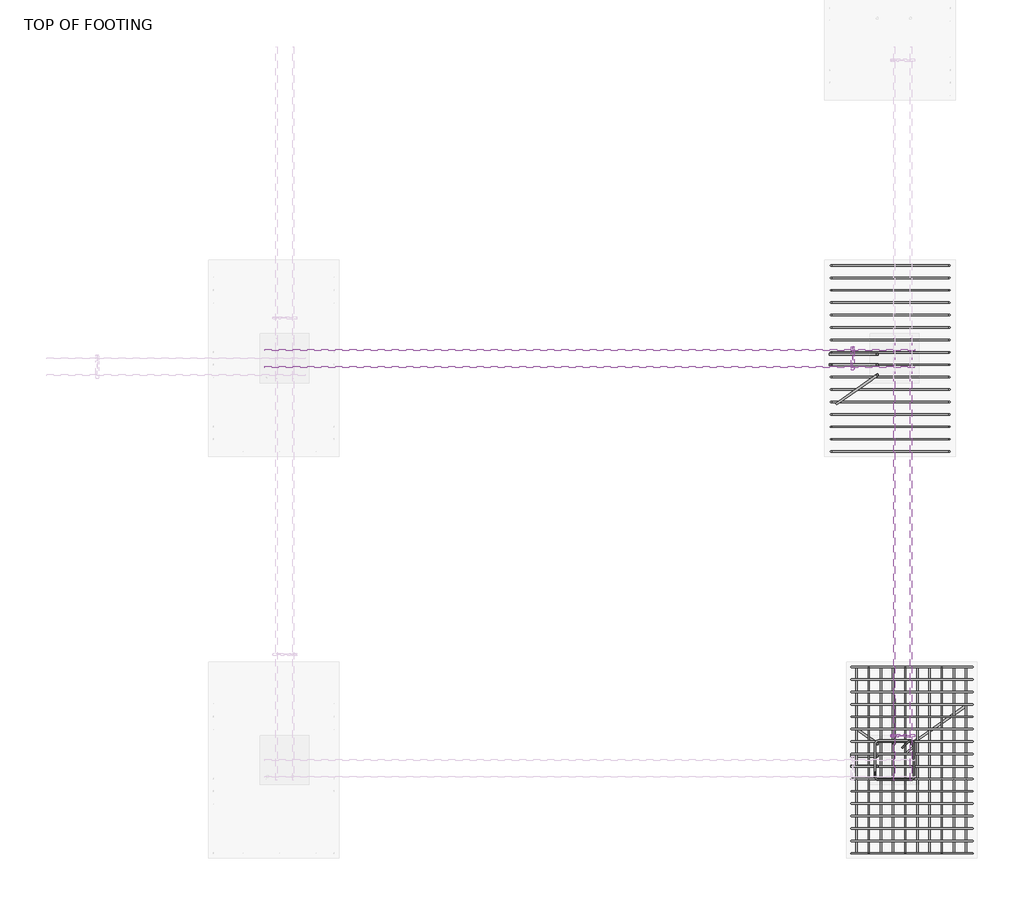
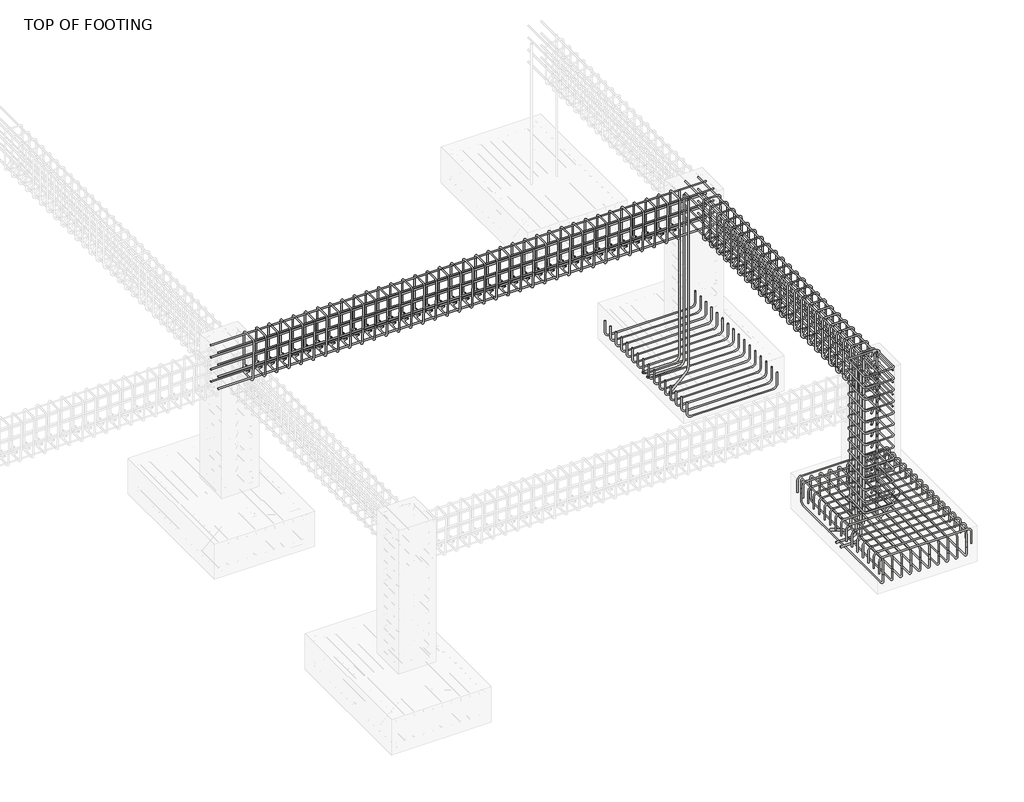
# One storey, part 5 of 11: 17 reinforcing bars.
"""IFC4 building model written with IfcOpenShell, lengths in millimetres."""

from ifc_helpers import new_model, si_unit, point, frame, origin, place, context, project, spatial, polyline, circle_curve, trimmed, segment, composite_curve, source, transform, mapped, element, save
from ifc_brep_helpers import swept_disk

model = new_model("IFC4")

# Units and contexts
model_context = context("Model", 3, world=origin())
ifc_project = project(units=[si_unit("LENGTHUNIT", "METRE", prefix="MILLI")], contexts=[model_context])

# Site, building, storey
site = spatial("IfcSite", under=ifc_project)
building = spatial("IfcBuilding", under=site)
storey = spatial("IfcBuildingStorey", under=building, Name="TOP OF FOOTING", Elevation=-1828.8)

# Reinforcing bars
placement = place(None, origin())
reinforcing_bar_shape = source(origin(), model_context, "Body", "SolidModel", [
    swept_disk(composite_curve([segment(polyline([(2940.9771951, -6018.1250095, -2061.9958198), (2940.9771951, -6018.1250095, -1914.6958198)]), True, "CONTINUOUS"), segment(trimmed(circle_curve(frame((2987.3271951, -6018.1250095, -1914.6958198), z_axis=(0.0, 1.0, 0.0), x_axis=(-46.350000000000364, 0.0, 0.0)), 46.35), [point((2940.9771951, -6018.1250095, -1914.6958198))], [point((2987.3271951, -6018.1250095, -1868.3458198))], True, "CARTESIAN"), True, "CONTINUOUS"), segment(polyline([(2987.3271951, -6018.1250095, -1868.3458198), (4001.9271951, -6018.1250095, -1868.3458198)]), True, "CONTINUOUS"), segment(trimmed(circle_curve(frame((4001.9271951, -6018.1250095, -1914.6958198), z_axis=(0.0, 1.0, 0.0), x_axis=(0.0, 0.0, 46.34999999999991)), 46.35), [point((4001.9271951, -6018.1250095, -1868.3458198))], [point((4048.2771951, -6018.1250095, -1914.6958198))], True, "CARTESIAN"), True, "CONTINUOUS"), segment(polyline([(4048.2771951, -6018.1250095, -1914.6958198), (4048.2771951, -6018.1250095, -2061.9958198)]), True, "CONTINUOUS")], self_intersect=False), 6.35),
])
element("IfcReinforcingBar", 1, at=placement, inside=storey, context=model_context, shape_type="MappedRepresentation", body=[
    mapped(reinforcing_bar_shape, transform((0.0, 0.0, 0.0), x_axis=(1.0, 0.0, 0.0), y_axis=(0.0, 1.0, 0.0), z_axis=(0.0, 0.0, 1.0))),
    mapped(reinforcing_bar_shape, transform((0.0, -113.82, 0.0), x_axis=(1.0, 0.0, 0.0), y_axis=(0.0, 1.0, 0.0), z_axis=(0.0, 0.0, 1.0))),
    mapped(reinforcing_bar_shape, transform((0.0, -227.64, 0.0), x_axis=(1.0, 0.0, 0.0), y_axis=(0.0, 1.0, 0.0), z_axis=(0.0, 0.0, 1.0))),
    mapped(reinforcing_bar_shape, transform((0.0, -341.46, 0.0), x_axis=(1.0, 0.0, 0.0), y_axis=(0.0, 1.0, 0.0), z_axis=(0.0, 0.0, 1.0))),
    mapped(reinforcing_bar_shape, transform((0.0, -455.28, 0.0), x_axis=(1.0, 0.0, 0.0), y_axis=(0.0, 1.0, 0.0), z_axis=(0.0, 0.0, 1.0))),
    mapped(reinforcing_bar_shape, transform((0.0, -569.1, 0.0), x_axis=(1.0, 0.0, 0.0), y_axis=(0.0, 1.0, 0.0), z_axis=(0.0, 0.0, 1.0))),
    mapped(reinforcing_bar_shape, transform((0.0, -682.92, 0.0), x_axis=(1.0, 0.0, 0.0), y_axis=(0.0, 1.0, 0.0), z_axis=(0.0, 0.0, 1.0))),
    mapped(reinforcing_bar_shape, transform((0.0, -796.74, 0.0), x_axis=(1.0, 0.0, 0.0), y_axis=(0.0, 1.0, 0.0), z_axis=(0.0, 0.0, 1.0))),
    mapped(reinforcing_bar_shape, transform((0.0, -910.56, 0.0), x_axis=(1.0, 0.0, 0.0), y_axis=(0.0, 1.0, 0.0), z_axis=(0.0, 0.0, 1.0))),
    mapped(reinforcing_bar_shape, transform((0.0, -1024.38, 0.0), x_axis=(1.0, 0.0, 0.0), y_axis=(0.0, 1.0, 0.0), z_axis=(0.0, 0.0, 1.0))),
    mapped(reinforcing_bar_shape, transform((0.0, -1138.2, 0.0), x_axis=(1.0, 0.0, 0.0), y_axis=(0.0, 1.0, 0.0), z_axis=(0.0, 0.0, 1.0))),
    mapped(reinforcing_bar_shape, transform((0.0, -1252.02, 0.0), x_axis=(1.0, 0.0, 0.0), y_axis=(0.0, 1.0, 0.0), z_axis=(0.0, 0.0, 1.0))),
    mapped(reinforcing_bar_shape, transform((0.0, -1365.84, 0.0), x_axis=(1.0, 0.0, 0.0), y_axis=(0.0, 1.0, 0.0), z_axis=(0.0, 0.0, 1.0))),
    mapped(reinforcing_bar_shape, transform((0.0, -1479.66, 0.0), x_axis=(1.0, 0.0, 0.0), y_axis=(0.0, 1.0, 0.0), z_axis=(0.0, 0.0, 1.0))),
    mapped(reinforcing_bar_shape, transform((0.0, -1593.48, 0.0), x_axis=(1.0, 0.0, 0.0), y_axis=(0.0, 1.0, 0.0), z_axis=(0.0, 0.0, 1.0))),
    mapped(reinforcing_bar_shape, transform((0.0, -1707.3, 0.0), x_axis=(1.0, 0.0, 0.0), y_axis=(0.0, 1.0, 0.0), z_axis=(0.0, 0.0, 1.0))),
])
reinforcing_bar_2_shape = source(origin(), model_context, "Body", "SolidModel", [
    swept_disk(composite_curve([segment(polyline([(3990.0605428, -6018.1250095, -2084.0984403), (3990.0605428, -6018.1250095, -1936.7984403)]), True, "CONTINUOUS"), segment(trimmed(circle_curve(frame((3990.0605428, -6064.4750095, -1936.7984403), z_axis=(1.0, 0.0, 0.0), x_axis=(0.0, 46.350000000000364, 0.0)), 46.35), [point((3990.0605428, -6018.1250095, -1936.7984403))], [point((3990.0605428, -6064.4750095, -1890.4484403))], True, "CARTESIAN"), True, "CONTINUOUS"), segment(polyline([(3990.0605428, -6064.4750095, -1890.4484403), (3990.0605428, -7679.0750095, -1890.4484403)]), True, "CONTINUOUS"), segment(trimmed(circle_curve(frame((3990.0605428, -7679.0750095, -1936.7984403), z_axis=(1.0, 0.0, 0.0), x_axis=(0.0, 0.0, 46.350000000000136)), 46.35), [point((3990.0605428, -7679.0750095, -1890.4484403))], [point((3990.0605428, -7725.4250095, -1936.7984403))], True, "CARTESIAN"), True, "CONTINUOUS"), segment(polyline([(3990.0605428, -7725.4250095, -1936.7984403), (3990.0605428, -7725.4250095, -2084.0984403)]), True, "CONTINUOUS")], self_intersect=False), 6.35),
])
element("IfcReinforcingBar", 2, at=placement, inside=storey, context=model_context, shape_type="MappedRepresentation", body=[
    mapped(reinforcing_bar_2_shape, transform((0.0, 0.0, 0.0), x_axis=(1.0, 0.0, 0.0), y_axis=(0.0, 1.0, 0.0), z_axis=(0.0, 0.0, 1.0))),
    mapped(reinforcing_bar_2_shape, transform((-111.55177, 0.0, 0.0), x_axis=(1.0, 0.0, 0.0), y_axis=(0.0, 1.0, 0.0), z_axis=(0.0, 0.0, 1.0))),
    mapped(reinforcing_bar_2_shape, transform((-223.10354, 0.0, 0.0), x_axis=(1.0, 0.0, 0.0), y_axis=(0.0, 1.0, 0.0), z_axis=(0.0, 0.0, 1.0))),
    mapped(reinforcing_bar_2_shape, transform((-334.6553099, 0.0, 0.0), x_axis=(1.0, 0.0, 0.0), y_axis=(0.0, 1.0, 0.0), z_axis=(0.0, 0.0, 1.0))),
    mapped(reinforcing_bar_2_shape, transform((-446.2070799, 0.0, 0.0), x_axis=(1.0, 0.0, 0.0), y_axis=(0.0, 1.0, 0.0), z_axis=(0.0, 0.0, 1.0))),
    mapped(reinforcing_bar_2_shape, transform((-557.7588499, 0.0, 0.0), x_axis=(1.0, 0.0, 0.0), y_axis=(0.0, 1.0, 0.0), z_axis=(0.0, 0.0, 1.0))),
    mapped(reinforcing_bar_2_shape, transform((-669.3106199, 0.0, 0.0), x_axis=(1.0, 0.0, 0.0), y_axis=(0.0, 1.0, 0.0), z_axis=(0.0, 0.0, 1.0))),
    mapped(reinforcing_bar_2_shape, transform((-780.8623899, 0.0, 0.0), x_axis=(1.0, 0.0, 0.0), y_axis=(0.0, 1.0, 0.0), z_axis=(0.0, 0.0, 1.0))),
    mapped(reinforcing_bar_2_shape, transform((-892.4141599, 0.0, 0.0), x_axis=(1.0, 0.0, 0.0), y_axis=(0.0, 1.0, 0.0), z_axis=(0.0, 0.0, 1.0))),
    mapped(reinforcing_bar_2_shape, transform((-1003.9659298, 0.0, 0.0), x_axis=(1.0, 0.0, 0.0), y_axis=(0.0, 1.0, 0.0), z_axis=(0.0, 0.0, 1.0))),
])
reinforcing_bar_3_shape = source(origin(), model_context, "Body", "SolidModel", [
    swept_disk(composite_curve([segment(polyline([(2986.0946129, -6018.1250095, -2021.5298587), (2986.0946129, -6018.1250095, -2168.8298587)]), True, "CONTINUOUS"), segment(trimmed(circle_curve(frame((2986.0946129, -6064.4750095, -2168.8298587), z_axis=(-1.0, 0.0, 0.0), x_axis=(0.0, 46.350000000000364, 0.0)), 46.35), [point((2986.0946129, -6018.1250095, -2168.8298587))], [point((2986.0946129, -6064.4750095, -2215.1798587))], True, "CARTESIAN"), True, "CONTINUOUS"), segment(polyline([(2986.0946129, -6064.4750095, -2215.1798587), (2986.0946129, -7679.0750095, -2215.1798587)]), True, "CONTINUOUS"), segment(trimmed(circle_curve(frame((2986.0946129, -7679.0750095, -2168.8298587), z_axis=(-1.0, 0.0, 0.0), x_axis=(0.0, 0.0, -46.34999999999991)), 46.35), [point((2986.0946129, -7679.0750095, -2215.1798587))], [point((2986.0946129, -7725.4250095, -2168.8298587))], True, "CARTESIAN"), True, "CONTINUOUS"), segment(polyline([(2986.0946129, -7725.4250095, -2168.8298587), (2986.0946129, -7725.4250095, -2021.5298587)]), True, "CONTINUOUS")], self_intersect=False), 6.35),
])
element("IfcReinforcingBar", 3, at=placement, inside=storey, context=model_context, shape_type="MappedRepresentation", body=[
    mapped(reinforcing_bar_3_shape, transform((0.0, 0.0, 0.0), x_axis=(1.0, 0.0, 0.0), y_axis=(0.0, 1.0, 0.0), z_axis=(0.0, 0.0, 1.0))),
    mapped(reinforcing_bar_3_shape, transform((111.55177, 0.0, 0.0), x_axis=(1.0, 0.0, 0.0), y_axis=(0.0, 1.0, 0.0), z_axis=(0.0, 0.0, 1.0))),
    mapped(reinforcing_bar_3_shape, transform((223.10354, 0.0, 0.0), x_axis=(1.0, 0.0, 0.0), y_axis=(0.0, 1.0, 0.0), z_axis=(0.0, 0.0, 1.0))),
    mapped(reinforcing_bar_3_shape, transform((334.6553099, 0.0, 0.0), x_axis=(1.0, 0.0, 0.0), y_axis=(0.0, 1.0, 0.0), z_axis=(0.0, 0.0, 1.0))),
    mapped(reinforcing_bar_3_shape, transform((446.2070799, 0.0, 0.0), x_axis=(1.0, 0.0, 0.0), y_axis=(0.0, 1.0, 0.0), z_axis=(0.0, 0.0, 1.0))),
    mapped(reinforcing_bar_3_shape, transform((557.7588499, 0.0, 0.0), x_axis=(1.0, 0.0, 0.0), y_axis=(0.0, 1.0, 0.0), z_axis=(0.0, 0.0, 1.0))),
    mapped(reinforcing_bar_3_shape, transform((669.3106199, 0.0, 0.0), x_axis=(1.0, 0.0, 0.0), y_axis=(0.0, 1.0, 0.0), z_axis=(0.0, 0.0, 1.0))),
    mapped(reinforcing_bar_3_shape, transform((780.8623899, 0.0, 0.0), x_axis=(1.0, 0.0, 0.0), y_axis=(0.0, 1.0, 0.0), z_axis=(0.0, 0.0, 1.0))),
    mapped(reinforcing_bar_3_shape, transform((892.4141599, 0.0, 0.0), x_axis=(1.0, 0.0, 0.0), y_axis=(0.0, 1.0, 0.0), z_axis=(0.0, 0.0, 1.0))),
    mapped(reinforcing_bar_3_shape, transform((1003.9659298, 0.0, 0.0), x_axis=(1.0, 0.0, 0.0), y_axis=(0.0, 1.0, 0.0), z_axis=(0.0, 0.0, 1.0))),
])
reinforcing_bar_4_shape = source(origin(), model_context, "Body", "SolidModel", [
    swept_disk(composite_curve([segment(polyline([(3836.7789753, -2335.4013044, -2046.7466921), (3836.7789753, -2335.4013044, -2194.0466921)]), True, "CONTINUOUS"), segment(trimmed(circle_curve(frame((3790.4289753, -2335.4013044, -2194.0466921), z_axis=(0.0, 1.0, 0.0), x_axis=(46.350000000000364, 0.0, 0.0)), 46.35), [point((3836.7789753, -2335.4013044, -2194.0466921))], [point((3790.4289753, -2335.4013044, -2240.3966921))], True, "CARTESIAN"), True, "CONTINUOUS"), segment(polyline([(3790.4289753, -2335.4013044, -2240.3966921), (2799.2007226, -2335.4013044, -2240.3966921)]), True, "CONTINUOUS"), segment(trimmed(circle_curve(frame((2799.2007226, -2335.4013044, -2194.0466921), z_axis=(0.0, 1.0, 0.0), x_axis=(0.0, 0.0, -46.34999999999991)), 46.35), [point((2799.2007226, -2335.4013044, -2240.3966921))], [point((2752.8507226, -2335.4013044, -2194.0466921))], True, "CARTESIAN"), True, "CONTINUOUS"), segment(polyline([(2752.8507226, -2335.4013044, -2194.0466921), (2752.8507226, -2335.4013044, -2046.7466921)]), True, "CONTINUOUS")], self_intersect=False), 6.35),
])
element("IfcReinforcingBar", 4, at=placement, inside=storey, context=model_context, shape_type="MappedRepresentation", body=[
    mapped(reinforcing_bar_4_shape, transform((0.0, 0.0, 0.0), x_axis=(1.0, 0.0, 0.0), y_axis=(0.0, 1.0, 0.0), z_axis=(0.0, 0.0, 1.0))),
    mapped(reinforcing_bar_4_shape, transform((0.0, -113.82, 0.0), x_axis=(1.0, 0.0, 0.0), y_axis=(0.0, 1.0, 0.0), z_axis=(0.0, 0.0, 1.0))),
    mapped(reinforcing_bar_4_shape, transform((0.0, -227.64, 0.0), x_axis=(1.0, 0.0, 0.0), y_axis=(0.0, 1.0, 0.0), z_axis=(0.0, 0.0, 1.0))),
    mapped(reinforcing_bar_4_shape, transform((0.0, -341.46, 0.0), x_axis=(1.0, 0.0, 0.0), y_axis=(0.0, 1.0, 0.0), z_axis=(0.0, 0.0, 1.0))),
    mapped(reinforcing_bar_4_shape, transform((0.0, -455.28, 0.0), x_axis=(1.0, 0.0, 0.0), y_axis=(0.0, 1.0, 0.0), z_axis=(0.0, 0.0, 1.0))),
    mapped(reinforcing_bar_4_shape, transform((0.0, -569.1, 0.0), x_axis=(1.0, 0.0, 0.0), y_axis=(0.0, 1.0, 0.0), z_axis=(0.0, 0.0, 1.0))),
    mapped(reinforcing_bar_4_shape, transform((0.0, -682.92, 0.0), x_axis=(1.0, 0.0, 0.0), y_axis=(0.0, 1.0, 0.0), z_axis=(0.0, 0.0, 1.0))),
    mapped(reinforcing_bar_4_shape, transform((0.0, -796.74, 0.0), x_axis=(1.0, 0.0, 0.0), y_axis=(0.0, 1.0, 0.0), z_axis=(0.0, 0.0, 1.0))),
    mapped(reinforcing_bar_4_shape, transform((0.0, -910.56, 0.0), x_axis=(1.0, 0.0, 0.0), y_axis=(0.0, 1.0, 0.0), z_axis=(0.0, 0.0, 1.0))),
    mapped(reinforcing_bar_4_shape, transform((0.0, -1024.38, 0.0), x_axis=(1.0, 0.0, 0.0), y_axis=(0.0, 1.0, 0.0), z_axis=(0.0, 0.0, 1.0))),
    mapped(reinforcing_bar_4_shape, transform((0.0, -1138.2, 0.0), x_axis=(1.0, 0.0, 0.0), y_axis=(0.0, 1.0, 0.0), z_axis=(0.0, 0.0, 1.0))),
    mapped(reinforcing_bar_4_shape, transform((0.0, -1252.02, 0.0), x_axis=(1.0, 0.0, 0.0), y_axis=(0.0, 1.0, 0.0), z_axis=(0.0, 0.0, 1.0))),
    mapped(reinforcing_bar_4_shape, transform((0.0, -1365.84, 0.0), x_axis=(1.0, 0.0, 0.0), y_axis=(0.0, 1.0, 0.0), z_axis=(0.0, 0.0, 1.0))),
    mapped(reinforcing_bar_4_shape, transform((0.0, -1479.66, 0.0), x_axis=(1.0, 0.0, 0.0), y_axis=(0.0, 1.0, 0.0), z_axis=(0.0, 0.0, 1.0))),
    mapped(reinforcing_bar_4_shape, transform((0.0, -1593.48, 0.0), x_axis=(1.0, 0.0, 0.0), y_axis=(0.0, 1.0, 0.0), z_axis=(0.0, 0.0, 1.0))),
    mapped(reinforcing_bar_4_shape, transform((0.0, -1707.3, 0.0), x_axis=(1.0, 0.0, 0.0), y_axis=(0.0, 1.0, 0.0), z_axis=(0.0, 0.0, 1.0))),
])
reinforcing_bar_5_shape = source(origin(), model_context, "Body", "SolidModel", [
    swept_disk(composite_curve([segment(polyline([(3404.0158346, -6758.0507749, -46.35), (3459.7593975, -6702.3072119, -46.35)]), True, "CONTINUOUS"), segment(trimmed(circle_curve(frame((3481.9271951, -6724.4750095, -46.35), z_axis=(0.0, 0.0, -1.0), x_axis=(-22.167797600000085, 22.167797600000085, 0.0)), 31.35), [point((3459.7593975, -6702.3072119, -46.35))], [point((3513.2771951, -6724.4750095, -46.35))], True, "CARTESIAN"), True, "CONTINUOUS"), segment(polyline([(3513.2771951, -6724.4750095, -46.35), (3513.2771951, -7019.0750095, -46.35)]), True, "CONTINUOUS"), segment(trimmed(circle_curve(frame((3481.9271951, -7019.0750095, -46.35), z_axis=(0.0, 0.0, -1.0), x_axis=(31.34999999999991, 0.0, 0.0)), 31.35), [point((3513.2771951, -7019.0750095, -46.35))], [point((3481.9271951, -7050.4250095, -46.35))], True, "CARTESIAN"), True, "CONTINUOUS"), segment(polyline([(3481.9271951, -7050.4250095, -46.35), (3187.3271951, -7050.4250095, -46.35)]), True, "CONTINUOUS"), segment(trimmed(circle_curve(frame((3187.3271951, -7019.0947946, -45.2363875), z_axis=(0.0, 0.03552192833448212, -0.9993688971583016), x_axis=(0.0, -31.3302149000001, -1.1136125000000021)), 31.35), [point((3187.3271951, -7050.4250095, -46.35))], [point((3155.9771951, -7019.0947946, -45.2363875))], True, "CARTESIAN"), True, "CONTINUOUS"), segment(polyline([(3155.9771951, -7019.0947946, -45.2363875), (3155.9771951, -6724.4552244, -34.7636125)]), True, "CONTINUOUS"), segment(trimmed(circle_curve(frame((3187.3271951, -6724.4552244, -34.7636125), z_axis=(0.0, 0.03552192833448212, -0.9993688971583016), x_axis=(-31.350000000000364, 0.0, 0.0)), 31.35), [point((3155.9771951, -6724.4552244, -34.7636125))], [point((3187.3271951, -6693.1250095, -33.65))], True, "CARTESIAN"), True, "CONTINUOUS"), segment(polyline([(3187.3271951, -6693.1250095, -33.65), (3481.9271951, -6693.1250095, -33.65)]), True, "CONTINUOUS"), segment(trimmed(circle_curve(frame((3481.9271951, -6724.4750095, -33.65), z_axis=(0.0, 0.0, -1.0), x_axis=(0.0, 31.350000000000364, 0.0)), 31.35), [point((3481.9271951, -6693.1250095, -33.65))], [point((3504.0949927, -6746.6428071, -33.65))], True, "CARTESIAN"), True, "CONTINUOUS"), segment(polyline([(3504.0949927, -6746.6428071, -33.65), (3448.3514297, -6802.3863701, -33.65)]), True, "CONTINUOUS")], self_intersect=False), 6.35),
])
element("IfcReinforcingBar", 5, at=placement, inside=storey, context=model_context, shape_type="MappedRepresentation", body=[
    mapped(reinforcing_bar_5_shape, transform((0.0, 0.0, 0.0), x_axis=(1.0, 0.0, 0.0), y_axis=(0.0, 1.0, 0.0), z_axis=(0.0, 0.0, 1.0))),
    mapped(reinforcing_bar_5_shape, transform((0.0, 0.0, -144.675), x_axis=(1.0, 0.0, 0.0), y_axis=(0.0, 1.0, 0.0), z_axis=(0.0, 0.0, 1.0))),
    mapped(reinforcing_bar_5_shape, transform((0.0, 0.0, -289.35), x_axis=(1.0, 0.0, 0.0), y_axis=(0.0, 1.0, 0.0), z_axis=(0.0, 0.0, 1.0))),
    mapped(reinforcing_bar_5_shape, transform((0.0, 0.0, -434.025), x_axis=(1.0, 0.0, 0.0), y_axis=(0.0, 1.0, 0.0), z_axis=(0.0, 0.0, 1.0))),
    mapped(reinforcing_bar_5_shape, transform((0.0, 0.0, -578.7), x_axis=(1.0, 0.0, 0.0), y_axis=(0.0, 1.0, 0.0), z_axis=(0.0, 0.0, 1.0))),
    mapped(reinforcing_bar_5_shape, transform((0.0, 0.0, -723.375), x_axis=(1.0, 0.0, 0.0), y_axis=(0.0, 1.0, 0.0), z_axis=(0.0, 0.0, 1.0))),
    mapped(reinforcing_bar_5_shape, transform((0.0, 0.0, -868.05), x_axis=(1.0, 0.0, 0.0), y_axis=(0.0, 1.0, 0.0), z_axis=(0.0, 0.0, 1.0))),
    mapped(reinforcing_bar_5_shape, transform((0.0, 0.0, -1012.725), x_axis=(1.0, 0.0, 0.0), y_axis=(0.0, 1.0, 0.0), z_axis=(0.0, 0.0, 1.0))),
    mapped(reinforcing_bar_5_shape, transform((0.0, 0.0, -1157.4), x_axis=(1.0, 0.0, 0.0), y_axis=(0.0, 1.0, 0.0), z_axis=(0.0, 0.0, 1.0))),
    mapped(reinforcing_bar_5_shape, transform((0.0, 0.0, -1302.075), x_axis=(1.0, 0.0, 0.0), y_axis=(0.0, 1.0, 0.0), z_axis=(0.0, 0.0, 1.0))),
    mapped(reinforcing_bar_5_shape, transform((0.0, 0.0, -1446.75), x_axis=(1.0, 0.0, 0.0), y_axis=(0.0, 1.0, 0.0), z_axis=(0.0, 0.0, 1.0))),
    mapped(reinforcing_bar_5_shape, transform((0.0, 0.0, -1591.425), x_axis=(1.0, 0.0, 0.0), y_axis=(0.0, 1.0, 0.0), z_axis=(0.0, 0.0, 1.0))),
    mapped(reinforcing_bar_5_shape, transform((0.0, 0.0, -1736.1), x_axis=(1.0, 0.0, 0.0), y_axis=(0.0, 1.0, 0.0), z_axis=(0.0, 0.0, 1.0))),
])
element("IfcReinforcingBar", 6, at=placement, inside=storey, context=model_context, shape_type="SolidModel", body=[
    swept_disk(composite_curve([segment(polyline([(3491.9271951, -6720.8250095, -40.0), (3491.9271951, -6720.8250095, -2136.75)]), True, "CONTINUOUS"), segment(trimmed(circle_curve(frame((3546.8513397, -6682.3667095, -2136.75), z_axis=(0.5735764363510477, -0.8191520442889907, 0.0), x_axis=(-54.92414460000009, -38.458300000000236, 0.0)), 67.05), [point((3491.9271951, -6720.8250095, -2136.75))], [point((3546.8513397, -6682.3667095, -2203.8))], True, "CARTESIAN"), True, "CONTINUOUS"), segment(polyline([(3546.8513397, -6682.3667095, -2203.8), (3989.9912438, -6372.0768081, -2203.8)]), True, "CONTINUOUS")], self_intersect=False), 9.55),
])
element("IfcReinforcingBar", 7, at=placement, inside=storey, context=model_context, shape_type="SolidModel", body=[
    swept_disk(composite_curve([segment(polyline([(3177.3271951, -6720.8250095, -40.0), (3177.3271951, -6720.8250095, -2136.75)]), True, "CONTINUOUS"), segment(trimmed(circle_curve(frame((3122.4030505, -6682.3667095, -2136.75), z_axis=(0.5735764363510478, 0.8191520442889907, 0.0), x_axis=(54.92414460000009, -38.458300000000236, 0.0)), 67.05), [point((3177.3271951, -6720.8250095, -2136.75))], [point((3122.4030505, -6682.3667095, -2203.8))], True, "CARTESIAN"), True, "CONTINUOUS"), segment(polyline([(3122.4030505, -6682.3667095, -2203.8), (2999.2631464, -6596.1432204, -2203.8)]), True, "CONTINUOUS")], self_intersect=False), 9.55),
])
reinforcing_bar_6_shape = source(origin(), model_context, "Body", "SolidModel", [
    swept_disk(composite_curve([segment(polyline([(3177.3271951, -6833.1823983, -40.0), (3177.3271951, -6833.1823983, -2136.75)]), True, "CONTINUOUS"), segment(trimmed(circle_curve(frame((3110.2771951, -6833.1823983, -2136.75), z_axis=(0.0, 1.0, 0.0), x_axis=(67.05000000000018, 0.0, 0.0)), 67.05), [point((3177.3271951, -6833.1823983, -2136.75))], [point((3110.2771951, -6833.1823983, -2203.8))], True, "CARTESIAN"), True, "CONTINUOUS"), segment(polyline([(3110.2771951, -6833.1823983, -2203.8), (2934.6271951, -6833.1823983, -2203.8)]), True, "CONTINUOUS")], self_intersect=False), 9.55),
])
element("IfcReinforcingBar", 8, at=placement, inside=storey, context=model_context, shape_type="MappedRepresentation", body=[
    mapped(reinforcing_bar_6_shape, transform((0.0, 0.0, 0.0), x_axis=(1.0, 0.0, 0.0), y_axis=(0.0, 1.0, 0.0), z_axis=(0.0, 0.0, 1.0))),
    mapped(reinforcing_bar_6_shape, transform((0.0, -94.3634327, 0.0), x_axis=(1.0, 0.0, 0.0), y_axis=(0.0, 1.0, 0.0), z_axis=(0.0, 0.0, 1.0))),
])
element("IfcReinforcingBar", 9, at=placement, inside=storey, context=model_context, shape_type="SolidModel", body=[
    swept_disk(composite_curve([segment(polyline([(3331.9271951, -6720.8250095, -40.0), (3331.9271951, -6720.8250095, -2136.75)]), True, "CONTINUOUS"), segment(trimmed(circle_curve(frame((3331.9271951, -6653.7750095, -2136.75), z_axis=(1.0, 0.0, 0.0), x_axis=(0.0, -67.05000000000018, 0.0)), 67.05), [point((3331.9271951, -6720.8250095, -2136.75))], [point((3331.9271951, -6653.7750095, -2203.8))], True, "CARTESIAN"), True, "CONTINUOUS"), segment(polyline([(3331.9271951, -6653.7750095, -2203.8), (3331.9271951, -6308.1250095, -2203.8)]), True, "CONTINUOUS")], self_intersect=False), 9.55),
])
element("IfcReinforcingBar", 10, at=placement, inside=storey, context=model_context, shape_type="SolidModel", body=[
    swept_disk(composite_curve([segment(polyline([(3177.3271951, -3340.0013044, -40.0), (3177.3271951, -3340.0013044, -2136.75)]), True, "CONTINUOUS"), segment(trimmed(circle_curve(frame((3122.4030505, -3378.4596044, -2136.75), z_axis=(-0.5735764363510477, 0.8191520442889907, 0.0), x_axis=(54.92414460000009, 38.45829999999978, 0.0)), 67.05), [point((3177.3271951, -3340.0013044, -2136.75))], [point((3122.4030505, -3378.4596044, -2203.8))], True, "CARTESIAN"), True, "CONTINUOUS"), segment(polyline([(3122.4030505, -3378.4596044, -2203.8), (2799.2631464, -3604.7246012, -2203.8)]), True, "CONTINUOUS")], self_intersect=False), 9.55),
])
reinforcing_bar_7_shape = source(origin(), model_context, "Body", "SolidModel", [
    swept_disk(composite_curve([segment(polyline([(3177.3271951, -3150.4586931, -40.0), (3177.3271951, -3150.4586931, -2136.75)]), True, "CONTINUOUS"), segment(trimmed(circle_curve(frame((3110.2771951, -3150.4586931, -2136.75), z_axis=(0.0, 1.0, 0.0), x_axis=(67.05000000000018, 0.0, 0.0)), 67.05), [point((3177.3271951, -3150.4586931, -2136.75))], [point((3110.2771951, -3150.4586931, -2203.8))], True, "CARTESIAN"), True, "CONTINUOUS"), segment(polyline([(3110.2771951, -3150.4586931, -2203.8), (2734.6271951, -3150.4586931, -2203.8)]), True, "CONTINUOUS")], self_intersect=False), 9.55),
])
element("IfcReinforcingBar", 11, at=placement, inside=storey, context=model_context, shape_type="MappedRepresentation", body=[
    mapped(reinforcing_bar_7_shape, transform((0.0, 0.0, 0.0), x_axis=(1.0, 0.0, 0.0), y_axis=(0.0, 1.0, 0.0), z_axis=(0.0, 0.0, 1.0))),
    mapped(reinforcing_bar_7_shape, transform((0.0, -94.3634327, 0.0), x_axis=(1.0, 0.0, 0.0), y_axis=(0.0, 1.0, 0.0), z_axis=(0.0, 0.0, 1.0))),
])
reinforcing_bar_8_shape = source(origin(), model_context, "Body", "SolidModel", [
    swept_disk(composite_curve([segment(polyline([(3415.2385556, -6640.4250095, -488.7242346), (3359.4949927, -6640.4250095, -544.4677976)]), True, "CONTINUOUS"), segment(trimmed(circle_curve(frame((3337.3271951, -6640.4250095, -522.3), z_axis=(0.0, 1.0, 0.0), x_axis=(22.16779759999963, 0.0, -22.167797600000085)), 31.35), [point((3359.4949927, -6640.4250095, -544.4677976))], [point((3305.9771951, -6640.4250095, -522.3))], True, "CARTESIAN"), True, "CONTINUOUS"), segment(polyline([(3305.9771951, -6640.4250095, -522.3), (3305.9771951, -6640.4250095, -77.7)]), True, "CONTINUOUS"), segment(trimmed(circle_curve(frame((3337.3271951, -6640.4250095, -77.7), z_axis=(0.0, 1.0, 0.0), x_axis=(-31.350000000000364, 0.0, 0.0)), 31.35), [point((3305.9771951, -6640.4250095, -77.7))], [point((3337.3271951, -6640.4250095, -46.35))], True, "CARTESIAN"), True, "CONTINUOUS"), segment(polyline([(3337.3271951, -6640.4250095, -46.35), (3481.9271951, -6640.4250095, -46.35)]), True, "CONTINUOUS"), segment(trimmed(circle_curve(frame((3481.9271951, -6641.2095952, -77.6901807), z_axis=(0.0, 0.9996867842138424, -0.025026655153786322), x_axis=(0.0, 0.784585700000207, 31.340180699999998)), 31.35), [point((3481.9271951, -6640.4250095, -46.35))], [point((3513.2771951, -6641.2095952, -77.6901807))], True, "CARTESIAN"), True, "CONTINUOUS"), segment(polyline([(3513.2771951, -6641.2095952, -77.6901807), (3513.2771951, -6652.3404239, -522.3098193)]), True, "CONTINUOUS"), segment(trimmed(circle_curve(frame((3481.9271951, -6652.3404239, -522.3098193), z_axis=(0.0, 0.9996867842138424, -0.025026655153786322), x_axis=(31.34999999999991, 0.0, 0.0)), 31.35), [point((3513.2771951, -6652.3404239, -522.3098193))], [point((3481.9271951, -6653.1250095, -553.65))], True, "CARTESIAN"), True, "CONTINUOUS"), segment(polyline([(3481.9271951, -6653.1250095, -553.65), (3337.3271951, -6653.1250095, -553.65)]), True, "CONTINUOUS"), segment(trimmed(circle_curve(frame((3337.3271951, -6653.1250095, -522.3), z_axis=(0.0, 1.0, 0.0), x_axis=(0.0, 0.0, -31.350000000000023)), 31.35), [point((3337.3271951, -6653.1250095, -553.65))], [point((3315.1593975, -6653.1250095, -500.1322024))], True, "CARTESIAN"), True, "CONTINUOUS"), segment(polyline([(3315.1593975, -6653.1250095, -500.1322024), (3370.9029605, -6653.1250095, -444.3886395)]), True, "CONTINUOUS")], self_intersect=False), 6.35),
])
element("IfcReinforcingBar", 12, at=placement, inside=storey, context=model_context, shape_type="MappedRepresentation", body=[
    mapped(reinforcing_bar_8_shape, transform((0.0, 0.0, 0.0), x_axis=(1.0, 0.0, 0.0), y_axis=(0.0, 1.0, 0.0), z_axis=(0.0, 0.0, 1.0))),
    mapped(reinforcing_bar_8_shape, transform((0.0, 146.3647139, 0.0), x_axis=(1.0, 0.0, 0.0), y_axis=(0.0, 1.0, 0.0), z_axis=(0.0, 0.0, 1.0))),
    mapped(reinforcing_bar_8_shape, transform((0.0, 292.7294277, 0.0), x_axis=(1.0, 0.0, 0.0), y_axis=(0.0, 1.0, 0.0), z_axis=(0.0, 0.0, 1.0))),
    mapped(reinforcing_bar_8_shape, transform((0.0, 439.0941416, 0.0), x_axis=(1.0, 0.0, 0.0), y_axis=(0.0, 1.0, 0.0), z_axis=(0.0, 0.0, 1.0))),
    mapped(reinforcing_bar_8_shape, transform((0.0, 585.4588555, 0.0), x_axis=(1.0, 0.0, 0.0), y_axis=(0.0, 1.0, 0.0), z_axis=(0.0, 0.0, 1.0))),
    mapped(reinforcing_bar_8_shape, transform((0.0, 731.8235693, 0.0), x_axis=(1.0, 0.0, 0.0), y_axis=(0.0, 1.0, 0.0), z_axis=(0.0, 0.0, 1.0))),
    mapped(reinforcing_bar_8_shape, transform((0.0, 878.1882832, 0.0), x_axis=(1.0, 0.0, 0.0), y_axis=(0.0, 1.0, 0.0), z_axis=(0.0, 0.0, 1.0))),
    mapped(reinforcing_bar_8_shape, transform((0.0, 1024.5529971, 0.0), x_axis=(1.0, 0.0, 0.0), y_axis=(0.0, 1.0, 0.0), z_axis=(0.0, 0.0, 1.0))),
    mapped(reinforcing_bar_8_shape, transform((0.0, 1170.917711, 0.0), x_axis=(1.0, 0.0, 0.0), y_axis=(0.0, 1.0, 0.0), z_axis=(0.0, 0.0, 1.0))),
    mapped(reinforcing_bar_8_shape, transform((0.0, 1317.2824248, 0.0), x_axis=(1.0, 0.0, 0.0), y_axis=(0.0, 1.0, 0.0), z_axis=(0.0, 0.0, 1.0))),
    mapped(reinforcing_bar_8_shape, transform((0.0, 1463.6471387, 0.0), x_axis=(1.0, 0.0, 0.0), y_axis=(0.0, 1.0, 0.0), z_axis=(0.0, 0.0, 1.0))),
    mapped(reinforcing_bar_8_shape, transform((0.0, 1610.0118526, 0.0), x_axis=(1.0, 0.0, 0.0), y_axis=(0.0, 1.0, 0.0), z_axis=(0.0, 0.0, 1.0))),
    mapped(reinforcing_bar_8_shape, transform((0.0, 1756.3765664, 0.0), x_axis=(1.0, 0.0, 0.0), y_axis=(0.0, 1.0, 0.0), z_axis=(0.0, 0.0, 1.0))),
    mapped(reinforcing_bar_8_shape, transform((0.0, 1902.7412803, 0.0), x_axis=(1.0, 0.0, 0.0), y_axis=(0.0, 1.0, 0.0), z_axis=(0.0, 0.0, 1.0))),
    mapped(reinforcing_bar_8_shape, transform((0.0, 2049.1059942, 0.0), x_axis=(1.0, 0.0, 0.0), y_axis=(0.0, 1.0, 0.0), z_axis=(0.0, 0.0, 1.0))),
    mapped(reinforcing_bar_8_shape, transform((0.0, 2195.470708, 0.0), x_axis=(1.0, 0.0, 0.0), y_axis=(0.0, 1.0, 0.0), z_axis=(0.0, 0.0, 1.0))),
    mapped(reinforcing_bar_8_shape, transform((0.0, 2341.8354219, 0.0), x_axis=(1.0, 0.0, 0.0), y_axis=(0.0, 1.0, 0.0), z_axis=(0.0, 0.0, 1.0))),
    mapped(reinforcing_bar_8_shape, transform((0.0, 2488.2001358, 0.0), x_axis=(1.0, 0.0, 0.0), y_axis=(0.0, 1.0, 0.0), z_axis=(0.0, 0.0, 1.0))),
    mapped(reinforcing_bar_8_shape, transform((0.0, 2634.5648497, 0.0), x_axis=(1.0, 0.0, 0.0), y_axis=(0.0, 1.0, 0.0), z_axis=(0.0, 0.0, 1.0))),
    mapped(reinforcing_bar_8_shape, transform((0.0, 2780.9295635, 0.0), x_axis=(1.0, 0.0, 0.0), y_axis=(0.0, 1.0, 0.0), z_axis=(0.0, 0.0, 1.0))),
    mapped(reinforcing_bar_8_shape, transform((0.0, 2927.2942774, 0.0), x_axis=(1.0, 0.0, 0.0), y_axis=(0.0, 1.0, 0.0), z_axis=(0.0, 0.0, 1.0))),
    mapped(reinforcing_bar_8_shape, transform((0.0, 3073.6589913, 0.0), x_axis=(1.0, 0.0, 0.0), y_axis=(0.0, 1.0, 0.0), z_axis=(0.0, 0.0, 1.0))),
    mapped(reinforcing_bar_8_shape, transform((0.0, 3220.0237051, 0.0), x_axis=(1.0, 0.0, 0.0), y_axis=(0.0, 1.0, 0.0), z_axis=(0.0, 0.0, 1.0))),
])
reinforcing_bar_9_shape = source(origin(), model_context, "Body", "SolidModel", [
    swept_disk(composite_curve([segment(polyline([(3332.3271951, -7056.7750095, -528.2977114), (3332.3271951, -3004.0513044, -528.2977114)]), True, "CONTINUOUS")], self_intersect=False), 6.35),
])
element("IfcReinforcingBar", 13, at=placement, inside=storey, context=model_context, shape_type="MappedRepresentation", body=[
    mapped(reinforcing_bar_9_shape, transform((0.0, 0.0, 0.0), x_axis=(1.0, 0.0, 0.0), y_axis=(0.0, 1.0, 0.0), z_axis=(0.0, 0.0, 1.0))),
    mapped(reinforcing_bar_9_shape, transform((0.0, 0.0, 153.3723948), x_axis=(1.0, 0.0, 0.0), y_axis=(0.0, 1.0, 0.0), z_axis=(0.0, 0.0, 1.0))),
    mapped(reinforcing_bar_9_shape, transform((0.0, 0.0, 306.7447895), x_axis=(1.0, 0.0, 0.0), y_axis=(0.0, 1.0, 0.0), z_axis=(0.0, 0.0, 1.0))),
    mapped(reinforcing_bar_9_shape, transform((0.0, 0.0, 460.1171843), x_axis=(1.0, 0.0, 0.0), y_axis=(0.0, 1.0, 0.0), z_axis=(0.0, 0.0, 1.0))),
])
reinforcing_bar_10_shape = source(origin(), model_context, "Body", "SolidModel", [
    swept_disk(composite_curve([segment(polyline([(3486.9271951, -7056.7750095, -528.2977114), (3486.9271951, -3004.0513044, -528.2977114)]), True, "CONTINUOUS")], self_intersect=False), 6.35),
])
element("IfcReinforcingBar", 14, at=placement, inside=storey, context=model_context, shape_type="MappedRepresentation", body=[
    mapped(reinforcing_bar_10_shape, transform((0.0, 0.0, 0.0), x_axis=(1.0, 0.0, 0.0), y_axis=(0.0, 1.0, 0.0), z_axis=(0.0, 0.0, 1.0))),
    mapped(reinforcing_bar_10_shape, transform((0.0, 0.0, 153.3723948), x_axis=(1.0, 0.0, 0.0), y_axis=(0.0, 1.0, 0.0), z_axis=(0.0, 0.0, 1.0))),
    mapped(reinforcing_bar_10_shape, transform((0.0, 0.0, 306.7447895), x_axis=(1.0, 0.0, 0.0), y_axis=(0.0, 1.0, 0.0), z_axis=(0.0, 0.0, 1.0))),
    mapped(reinforcing_bar_10_shape, transform((0.0, 0.0, 460.1171843), x_axis=(1.0, 0.0, 0.0), y_axis=(0.0, 1.0, 0.0), z_axis=(0.0, 0.0, 1.0))),
])
reinforcing_bar_11_shape = source(origin(), model_context, "Body", "SolidModel", [
    swept_disk(composite_curve([segment(polyline([(-2024.0228055, -3194.6626649, -488.7242346), (-2024.0228055, -3138.919102, -544.4677976)]), True, "CONTINUOUS"), segment(trimmed(circle_curve(frame((-2024.0228055, -3116.7513044, -522.3), z_axis=(1.0, 0.0, 0.0), x_axis=(0.0, -22.16779759999963, -22.167797600000085)), 31.35), [point((-2024.0228055, -3138.919102, -544.4677976))], [point((-2024.0228055, -3085.4013044, -522.3))], True, "CARTESIAN"), True, "CONTINUOUS"), segment(polyline([(-2024.0228055, -3085.4013044, -522.3), (-2024.0228055, -3085.4013044, -77.7)]), True, "CONTINUOUS"), segment(trimmed(circle_curve(frame((-2024.0228055, -3116.7513044, -77.7), z_axis=(1.0, 0.0, 0.0), x_axis=(0.0, 31.350000000000364, 0.0)), 31.35), [point((-2024.0228055, -3085.4013044, -77.7))], [point((-2024.0228055, -3116.7513044, -46.35))], True, "CARTESIAN"), True, "CONTINUOUS"), segment(polyline([(-2024.0228055, -3116.7513044, -46.35), (-2024.0228055, -3261.3513044, -46.35)]), True, "CONTINUOUS"), segment(trimmed(circle_curve(frame((-2024.8073911, -3261.3513044, -77.6901807), z_axis=(0.9996867842138424, 0.0, -0.025026655153786322), x_axis=(0.7845855999999003, 0.0, 31.340180699999998)), 31.35), [point((-2024.0228055, -3261.3513044, -46.35))], [point((-2024.8073911, -3292.7013044, -77.6901807))], True, "CARTESIAN"), True, "CONTINUOUS"), segment(polyline([(-2024.8073911, -3292.7013044, -77.6901807), (-2035.9382199, -3292.7013044, -522.3098193)]), True, "CONTINUOUS"), segment(trimmed(circle_curve(frame((-2035.9382199, -3261.3513044, -522.3098193), z_axis=(0.9996867842138424, 0.0, -0.025026655153786322), x_axis=(0.0, -31.34999999999991, 0.0)), 31.35), [point((-2035.9382199, -3292.7013044, -522.3098193))], [point((-2036.7228055, -3261.3513044, -553.65))], True, "CARTESIAN"), True, "CONTINUOUS"), segment(polyline([(-2036.7228055, -3261.3513044, -553.65), (-2036.7228055, -3116.7513044, -553.65)]), True, "CONTINUOUS"), segment(trimmed(circle_curve(frame((-2036.7228055, -3116.7513044, -522.3), z_axis=(1.0, 0.0, 0.0), x_axis=(0.0, 0.0, -31.350000000000023)), 31.35), [point((-2036.7228055, -3116.7513044, -553.65))], [point((-2036.7228055, -3094.5835068, -500.1322024))], True, "CARTESIAN"), True, "CONTINUOUS"), segment(polyline([(-2036.7228055, -3094.5835068, -500.1322024), (-2036.7228055, -3150.3270697, -444.3886395)]), True, "CONTINUOUS")], self_intersect=False), 6.35),
])
element("IfcReinforcingBar", 15, at=placement, inside=storey, context=model_context, shape_type="MappedRepresentation", body=[
    mapped(reinforcing_bar_11_shape, transform((0.0, 0.0, 0.0), x_axis=(1.0, 0.0, 0.0), y_axis=(0.0, 1.0, 0.0), z_axis=(0.0, 0.0, 1.0))),
    mapped(reinforcing_bar_11_shape, transform((146.4942857, 0.0, 0.0), x_axis=(1.0, 0.0, 0.0), y_axis=(0.0, 1.0, 0.0), z_axis=(0.0, 0.0, 1.0))),
    mapped(reinforcing_bar_11_shape, transform((292.9885715, 0.0, 0.0), x_axis=(1.0, 0.0, 0.0), y_axis=(0.0, 1.0, 0.0), z_axis=(0.0, 0.0, 1.0))),
    mapped(reinforcing_bar_11_shape, transform((439.4828572, 0.0, 0.0), x_axis=(1.0, 0.0, 0.0), y_axis=(0.0, 1.0, 0.0), z_axis=(0.0, 0.0, 1.0))),
    mapped(reinforcing_bar_11_shape, transform((585.9771429, 0.0, 0.0), x_axis=(1.0, 0.0, 0.0), y_axis=(0.0, 1.0, 0.0), z_axis=(0.0, 0.0, 1.0))),
    mapped(reinforcing_bar_11_shape, transform((732.4714287, 0.0, 0.0), x_axis=(1.0, 0.0, 0.0), y_axis=(0.0, 1.0, 0.0), z_axis=(0.0, 0.0, 1.0))),
    mapped(reinforcing_bar_11_shape, transform((878.9657144, 0.0, 0.0), x_axis=(1.0, 0.0, 0.0), y_axis=(0.0, 1.0, 0.0), z_axis=(0.0, 0.0, 1.0))),
    mapped(reinforcing_bar_11_shape, transform((1025.4600001, 0.0, 0.0), x_axis=(1.0, 0.0, 0.0), y_axis=(0.0, 1.0, 0.0), z_axis=(0.0, 0.0, 1.0))),
    mapped(reinforcing_bar_11_shape, transform((1171.9542859, 0.0, 0.0), x_axis=(1.0, 0.0, 0.0), y_axis=(0.0, 1.0, 0.0), z_axis=(0.0, 0.0, 1.0))),
    mapped(reinforcing_bar_11_shape, transform((1318.4485716, 0.0, 0.0), x_axis=(1.0, 0.0, 0.0), y_axis=(0.0, 1.0, 0.0), z_axis=(0.0, 0.0, 1.0))),
    mapped(reinforcing_bar_11_shape, transform((1464.9428573, 0.0, 0.0), x_axis=(1.0, 0.0, 0.0), y_axis=(0.0, 1.0, 0.0), z_axis=(0.0, 0.0, 1.0))),
    mapped(reinforcing_bar_11_shape, transform((1611.437143, 0.0, 0.0), x_axis=(1.0, 0.0, 0.0), y_axis=(0.0, 1.0, 0.0), z_axis=(0.0, 0.0, 1.0))),
    mapped(reinforcing_bar_11_shape, transform((1757.9314288, 0.0, 0.0), x_axis=(1.0, 0.0, 0.0), y_axis=(0.0, 1.0, 0.0), z_axis=(0.0, 0.0, 1.0))),
    mapped(reinforcing_bar_11_shape, transform((1904.4257145, 0.0, 0.0), x_axis=(1.0, 0.0, 0.0), y_axis=(0.0, 1.0, 0.0), z_axis=(0.0, 0.0, 1.0))),
    mapped(reinforcing_bar_11_shape, transform((2050.9200002, 0.0, 0.0), x_axis=(1.0, 0.0, 0.0), y_axis=(0.0, 1.0, 0.0), z_axis=(0.0, 0.0, 1.0))),
    mapped(reinforcing_bar_11_shape, transform((2197.414286, 0.0, 0.0), x_axis=(1.0, 0.0, 0.0), y_axis=(0.0, 1.0, 0.0), z_axis=(0.0, 0.0, 1.0))),
    mapped(reinforcing_bar_11_shape, transform((2343.9085717, 0.0, 0.0), x_axis=(1.0, 0.0, 0.0), y_axis=(0.0, 1.0, 0.0), z_axis=(0.0, 0.0, 1.0))),
    mapped(reinforcing_bar_11_shape, transform((2490.4028574, 0.0, 0.0), x_axis=(1.0, 0.0, 0.0), y_axis=(0.0, 1.0, 0.0), z_axis=(0.0, 0.0, 1.0))),
    mapped(reinforcing_bar_11_shape, transform((2636.8971432, 0.0, 0.0), x_axis=(1.0, 0.0, 0.0), y_axis=(0.0, 1.0, 0.0), z_axis=(0.0, 0.0, 1.0))),
    mapped(reinforcing_bar_11_shape, transform((2783.3914289, 0.0, 0.0), x_axis=(1.0, 0.0, 0.0), y_axis=(0.0, 1.0, 0.0), z_axis=(0.0, 0.0, 1.0))),
    mapped(reinforcing_bar_11_shape, transform((2929.8857146, 0.0, 0.0), x_axis=(1.0, 0.0, 0.0), y_axis=(0.0, 1.0, 0.0), z_axis=(0.0, 0.0, 1.0))),
    mapped(reinforcing_bar_11_shape, transform((3076.3800004, 0.0, 0.0), x_axis=(1.0, 0.0, 0.0), y_axis=(0.0, 1.0, 0.0), z_axis=(0.0, 0.0, 1.0))),
    mapped(reinforcing_bar_11_shape, transform((3222.8742861, 0.0, 0.0), x_axis=(1.0, 0.0, 0.0), y_axis=(0.0, 1.0, 0.0), z_axis=(0.0, 0.0, 1.0))),
    mapped(reinforcing_bar_11_shape, transform((3369.3685718, 0.0, 0.0), x_axis=(1.0, 0.0, 0.0), y_axis=(0.0, 1.0, 0.0), z_axis=(0.0, 0.0, 1.0))),
    mapped(reinforcing_bar_11_shape, transform((3515.8628576, 0.0, 0.0), x_axis=(1.0, 0.0, 0.0), y_axis=(0.0, 1.0, 0.0), z_axis=(0.0, 0.0, 1.0))),
    mapped(reinforcing_bar_11_shape, transform((3662.3571433, 0.0, 0.0), x_axis=(1.0, 0.0, 0.0), y_axis=(0.0, 1.0, 0.0), z_axis=(0.0, 0.0, 1.0))),
    mapped(reinforcing_bar_11_shape, transform((3808.851429, 0.0, 0.0), x_axis=(1.0, 0.0, 0.0), y_axis=(0.0, 1.0, 0.0), z_axis=(0.0, 0.0, 1.0))),
    mapped(reinforcing_bar_11_shape, transform((3955.3457148, 0.0, 0.0), x_axis=(1.0, 0.0, 0.0), y_axis=(0.0, 1.0, 0.0), z_axis=(0.0, 0.0, 1.0))),
    mapped(reinforcing_bar_11_shape, transform((4101.8400005, 0.0, 0.0), x_axis=(1.0, 0.0, 0.0), y_axis=(0.0, 1.0, 0.0), z_axis=(0.0, 0.0, 1.0))),
    mapped(reinforcing_bar_11_shape, transform((4248.3342862, 0.0, 0.0), x_axis=(1.0, 0.0, 0.0), y_axis=(0.0, 1.0, 0.0), z_axis=(0.0, 0.0, 1.0))),
    mapped(reinforcing_bar_11_shape, transform((4394.828572, 0.0, 0.0), x_axis=(1.0, 0.0, 0.0), y_axis=(0.0, 1.0, 0.0), z_axis=(0.0, 0.0, 1.0))),
    mapped(reinforcing_bar_11_shape, transform((4541.3228577, 0.0, 0.0), x_axis=(1.0, 0.0, 0.0), y_axis=(0.0, 1.0, 0.0), z_axis=(0.0, 0.0, 1.0))),
    mapped(reinforcing_bar_11_shape, transform((4687.8171434, 0.0, 0.0), x_axis=(1.0, 0.0, 0.0), y_axis=(0.0, 1.0, 0.0), z_axis=(0.0, 0.0, 1.0))),
    mapped(reinforcing_bar_11_shape, transform((4834.3114291, 0.0, 0.0), x_axis=(1.0, 0.0, 0.0), y_axis=(0.0, 1.0, 0.0), z_axis=(0.0, 0.0, 1.0))),
    mapped(reinforcing_bar_11_shape, transform((4980.8057149, 0.0, 0.0), x_axis=(1.0, 0.0, 0.0), y_axis=(0.0, 1.0, 0.0), z_axis=(0.0, 0.0, 1.0))),
    mapped(reinforcing_bar_11_shape, transform((5127.3000006, 0.0, 0.0), x_axis=(1.0, 0.0, 0.0), y_axis=(0.0, 1.0, 0.0), z_axis=(0.0, 0.0, 1.0))),
])
reinforcing_bar_12_shape = source(origin(), model_context, "Body", "SolidModel", [
    swept_disk(composite_curve([segment(polyline([(-2440.3728049, -3111.7513044, -528.2977114), (3519.6271951, -3111.7513044, -528.2977114)]), True, "CONTINUOUS")], self_intersect=False), 6.35),
])
element("IfcReinforcingBar", 16, at=placement, inside=storey, context=model_context, shape_type="MappedRepresentation", body=[
    mapped(reinforcing_bar_12_shape, transform((0.0, 0.0, 0.0), x_axis=(1.0, 0.0, 0.0), y_axis=(0.0, 1.0, 0.0), z_axis=(0.0, 0.0, 1.0))),
    mapped(reinforcing_bar_12_shape, transform((0.0, 0.0, 153.3723948), x_axis=(1.0, 0.0, 0.0), y_axis=(0.0, 1.0, 0.0), z_axis=(0.0, 0.0, 1.0))),
    mapped(reinforcing_bar_12_shape, transform((0.0, 0.0, 306.7447895), x_axis=(1.0, 0.0, 0.0), y_axis=(0.0, 1.0, 0.0), z_axis=(0.0, 0.0, 1.0))),
    mapped(reinforcing_bar_12_shape, transform((0.0, 0.0, 460.1171843), x_axis=(1.0, 0.0, 0.0), y_axis=(0.0, 1.0, 0.0), z_axis=(0.0, 0.0, 1.0))),
])
reinforcing_bar_13_shape = source(origin(), model_context, "Body", "SolidModel", [
    swept_disk(composite_curve([segment(polyline([(-2440.3728049, -3266.3513044, -528.2977114), (3519.6271951, -3266.3513044, -528.2977114)]), True, "CONTINUOUS")], self_intersect=False), 6.35),
])
element("IfcReinforcingBar", 17, at=placement, inside=storey, context=model_context, shape_type="MappedRepresentation", body=[
    mapped(reinforcing_bar_13_shape, transform((0.0, 0.0, 0.0), x_axis=(1.0, 0.0, 0.0), y_axis=(0.0, 1.0, 0.0), z_axis=(0.0, 0.0, 1.0))),
    mapped(reinforcing_bar_13_shape, transform((0.0, 0.0, 153.3723948), x_axis=(1.0, 0.0, 0.0), y_axis=(0.0, 1.0, 0.0), z_axis=(0.0, 0.0, 1.0))),
    mapped(reinforcing_bar_13_shape, transform((0.0, 0.0, 306.7447895), x_axis=(1.0, 0.0, 0.0), y_axis=(0.0, 1.0, 0.0), z_axis=(0.0, 0.0, 1.0))),
    mapped(reinforcing_bar_13_shape, transform((0.0, 0.0, 460.1171843), x_axis=(1.0, 0.0, 0.0), y_axis=(0.0, 1.0, 0.0), z_axis=(0.0, 0.0, 1.0))),
])

save(model, "model.ifc")

# Revit data of these elements
# Elements 1, 2, 3, 4, 5, 6, 7, 8, 9, 10, 11, 12, 13, 14, 15, 16, 17 (IfcReinforcingBar)
#   Phase Created = New Construction
